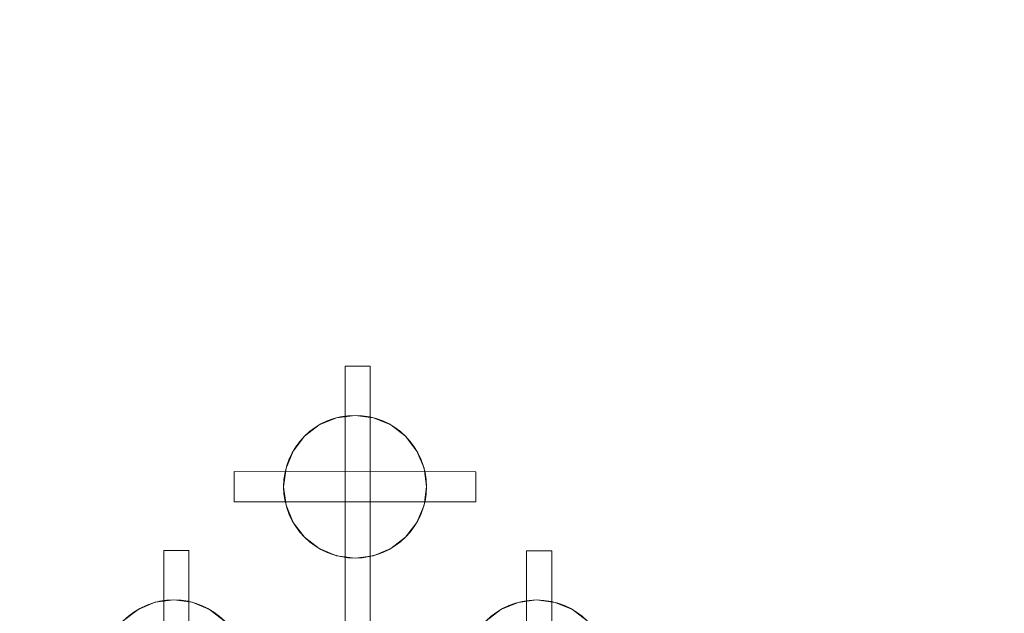
# Model space of a CAD drawing. Units: inches. Extents: x 2696 to 3240, y 1564 to 2310.
# Tile 71 of 76: x 3144.26 to 3156.48, y 2078.13 to 2085.5. Entities that reach past the tile are written whole.
import ezdxf

# ---------------------------------------------------------------- set-up
doc = ezdxf.new("R2010")
doc.units = ezdxf.units.IN
for name, color, linetype, lineweight in [('A-ANNO-DIMS', 3, 'Continuous', 18), ('A-FLOR-FIXT', 8, 'Continuous', 18), ('A-FURN', 251, 'Continuous', 13)]:
    doc.layers.add(name, color=color, linetype=linetype, lineweight=lineweight)
doc.layers.add('FURNITURE', color=250, linetype='Continuous')
doc.styles.add('TIMES NEW', font='times.ttf')
doc.dimstyles.new('Siddhuu', dxfattribs={"dimtxt": 6, "dimasz": 2.5, "dimexe": 1.25, "dimexo": 0.625, "dimtad": 1, "dimdec": 1, "dimlunit": 4, "dimtxsty": 'TIMES NEW', "dimcen": 2.5, "dimclrd": 256, "dimclre": 1, "dimclrt": 7, "dimadec": 0, "dimazin": 0, "dimtfac": 1, "dimtdec": 1, "dimtmove": 0, "dimatfit": 3, "dimfxl": 1, "dimtolj": 1, "dimlwd": -1, "dimarcsym": 0})

# ---------------------------------------------------------------- blocks, each defined once
blk = doc.blocks.new('A$C1af1f523')
at = {"layer": 'A-FURN'}
for p, q in [((-2.9, 3.935), (-2.9, 0.936)), ((-2.9, 3.935, 0.5), (-2.9, 0.936, 0.5)), ((-2.9, 3.935), (-2.9, 3.935, 0.5)), ((-2.525, 3.935), (-2.9, 3.935)), ((-2.525, 3.935, 0.5), (-2.9, 3.935, 0.5)), ((-2.525, 3.935), (-2.525, 0.936)), ((-2.525, 3.935, 0.5), (-2.525, 0.936, 0.5)), ((-2.525, 3.935), (-2.525, 3.935, 0.5)), ((-2.713, 3.321), (-2.713, 3.321, 0.5)), ((-3.156, 3.203), (-3.156, 3.203, 0.5)), ((-2.942, 3.291), (-2.942, 3.291, 0.5)), ((-2.483, 3.291), (-2.483, 3.291, 0.5)), ((-2.27, 3.203), (-2.27, 3.203, 0.5)), ((-3.339, 3.062), (-3.339, 3.062, 0.5)), ((-2.086, 3.062), (-2.086, 3.062, 0.5)), ((-3.48, 2.878), (-3.48, 2.878, 0.5)), ((-1.945, 2.878), (-1.945, 2.878, 0.5)), ((-3.569, 2.665), (-3.569, 2.665, 0.5)), ((-1.857, 2.665), (-1.857, 2.665, 0.5)), ((0, 2.56), (-4.212, 2.56)), ((0, 2.56, 0.5), (-4.212, 2.56, 0.5)), ((-4.212, 2.56), (-4.212, 2.56, 0.5)), ((-4.212, 2.559), (-4.212, 2.248)), ((-4.212, 2.559, 0.5), (-4.212, 2.248, 0.5)), ((-4.212, 2.559), (-4.212, 2.559, 0.5)), ((-3.599, 2.435), (-3.599, 2.435, 0.5)), ((-1.827, 2.435), (-1.827, 2.435, 0.5)), ((0, 2.248), (-4.212, 2.248)), ((0, 2.248, 0.5), (-4.212, 2.248, 0.5)), ((-4.212, 2.248), (-4.212, 2.248, 0.5)), ((-4.212, 2.248), (-4.212, 2.247)), ((-4.212, 2.248, 0.5), (-4.212, 2.247, 0.5)), ((-4.212, 2.247), (-4.212, 2.247, 0.5)), ((-3.569, 2.206), (-3.569, 2.206, 0.5)), ((-1.857, 2.206), (-1.857, 2.206, 0.5)), ((-3.48, 1.992), (-3.48, 1.992, 0.5)), ((-1.945, 1.992), (-1.945, 1.992, 0.5)), ((-3.339, 1.809), (-3.339, 1.809, 0.5)), ((-2.086, 1.809), (-2.086, 1.809, 0.5)), ((-4.816, 1.687), (-5.191, 1.687)), ((-4.816, 1.687, 0.5), (-5.191, 1.687, 0.5)), ((-5.191, 1.687), (-5.191, 1.687, 0.5)), ((-5.191, 1.687), (-5.19, -1.311)), ((-5.191, 1.687, 0.5), (-5.19, -1.311, 0.5)), ((-4.816, 1.687), (-4.816, 1.687, 0.5)), ((-4.816, 1.687), (-4.815, -1.311)), ((-4.816, 1.687, 0.5), (-4.815, -1.311, 0.5)), ((-3.156, 1.668), (-3.156, 1.668, 0.5)), ((-2.27, 1.668), (-2.27, 1.668, 0.5)), ((-2.942, 1.58), (-2.942, 1.58, 0.5)), ((-2.713, 1.549), (-2.713, 1.549, 0.5)), ((-2.483, 1.58), (-2.483, 1.58, 0.5)), ((-5.232, 1.043), (-5.232, 1.043, 0.5)), ((-5.003, 1.074), (-5.003, 1.074, 0.5)), ((-4.773, 1.043), (-4.773, 1.043, 0.5)), ((-5.446, 0.955), (-5.446, 0.955, 0.5)), ((-4.56, 0.955), (-4.56, 0.955, 0.5)), ((-2.9, 0.936), (-2.9, 0.936, 0.5)), ((-2.525, 0.936), (-2.898, 0.936)), ((-2.525, 0.936, 0.5), (-2.898, 0.936, 0.5)), ((-2.898, 0.936), (-2.898, 0.936, 0.5)), ((-2.525, 0.936), (-2.525, 0.936, 0.5)), ((-5.629, 0.814), (-5.629, 0.814, 0.5)), ((-4.376, 0.814), (-4.376, 0.814, 0.5)), ((-5.77, 0.631), (-5.77, 0.631, 0.5)), ((-4.235, 0.631), (-4.235, 0.631, 0.5)), ((-5.858, 0.417), (-5.858, 0.417, 0.5)), ((-4.147, 0.417), (-4.147, 0.417, 0.5)), ((0, 0.312), (-6.501, 0.312)), ((0, 0.312, 0.5), (-6.501, 0.312, 0.5)), ((-6.501, 0.312), (-6.501, 0.312, 0.5)), ((-6.501, 0.311), (-6.501, 0)), ((-6.501, 0.311, 0.5), (-6.501, 0, 0.5)), ((-6.501, 0.311), (-6.501, 0.311, 0.5)), ((-5.889, 0.188), (-5.889, 0.188, 0.5)), ((-4.117, 0.188), (-4.117, 0.188, 0.5)), ((0, 0), (-6.501, 0)), ((0, 0, 0.5), (-6.501, 0, 0.5)), ((-6.501, 0), (-6.501, 0, 0.5)), ((-6.501, 0), (-6.501, -0.001)), ((-6.501, 0, 0.5), (-6.501, -0.001, 0.5)), ((-6.501, -0.001), (-6.501, -0.001, 0.5)), ((-5.858, -0.042), (-5.858, -0.042, 0.5)), ((-4.147, -0.042), (-4.147, -0.042, 0.5)), ((-5.77, -0.256), (-5.77, -0.256, 0.5)), ((-4.235, -0.256), (-4.235, -0.256, 0.5)), ((-5.629, -0.439), (-5.629, -0.439, 0.5)), ((-4.376, -0.439), (-4.376, -0.439, 0.5)), ((-5.446, -0.58), (-5.446, -0.58, 0.5)), ((-4.56, -0.58), (-4.56, -0.58, 0.5)), ((-2.898, -0.564), (-2.898, -3.563)), ((-2.898, -0.564, 0.5), (-2.898, -3.563, 0.5)), ((-2.898, -0.564), (-2.898, -0.564, 0.5)), ((-2.523, -0.564), (-2.898, -0.564)), ((-2.523, -0.564, 0.5), (-2.898, -0.564, 0.5)), ((-2.523, -0.564), (-2.523, -3.563)), ((-2.523, -0.564, 0.5), (-2.523, -3.563, 0.5)), ((-2.523, -0.564), (-2.523, -0.564, 0.5)), ((-5.232, -0.668), (-5.232, -0.668, 0.5)), ((-5.003, -0.699), (-5.003, -0.699, 0.5)), ((-4.773, -0.668), (-4.773, -0.668, 0.5)), ((-2.94, -1.208), (-2.94, -1.208, 0.5)), ((-2.711, -1.178), (-2.711, -1.178, 0.5)), ((-2.481, -1.208), (-2.481, -1.208, 0.5)), ((-5.19, -1.311), (-5.19, -1.311, 0.5)), ((-4.815, -1.311), (-5.188, -1.311)), ((-4.815, -1.311, 0.5), (-5.188, -1.311, 0.5)), ((-5.188, -1.311), (-5.188, -1.311, 0.5)), ((-4.815, -1.311), (-4.815, -1.311, 0.5)), ((-3.154, -1.296), (-3.154, -1.296, 0.5)), ((-2.268, -1.296), (-2.268, -1.296, 0.5)), ((-3.337, -1.437), (-3.337, -1.437, 0.5)), ((-2.084, -1.437), (-2.084, -1.437, 0.5)), ((-3.478, -1.621), (-3.478, -1.621, 0.5)), ((-1.943, -1.621), (-1.943, -1.621, 0.5)), ((0, -1.939), (-4.209, -1.939)), ((0, -1.939, 0.5), (-4.209, -1.939, 0.5)), ((-4.209, -1.939), (-4.209, -1.939, 0.5)), ((-4.209, -1.94), (-4.209, -2.251)), ((-4.209, -1.94, 0.5), (-4.209, -2.251, 0.5)), ((-4.209, -1.94), (-4.209, -1.94, 0.5)), ((-3.566, -1.834), (-3.566, -1.834, 0.5)), ((-1.855, -1.834), (-1.855, -1.834, 0.5)), ((-3.597, -2.064), (-3.597, -2.064, 0.5)), ((-1.824, -2.064), (-1.824, -2.064, 0.5)), ((0, -2.251), (-4.209, -2.251)), ((0, -2.251, 0.5), (-4.209, -2.251, 0.5)), ((-4.209, -2.251), (-4.209, -2.251, 0.5)), ((-4.209, -2.251), (-4.209, -2.252)), ((-4.209, -2.251, 0.5), (-4.209, -2.252, 0.5)), ((-4.209, -2.252), (-4.209, -2.252, 0.5)), ((-3.566, -2.293), (-3.566, -2.293, 0.5)), ((-1.855, -2.293), (-1.855, -2.293, 0.5)), ((-3.478, -2.507), (-3.478, -2.507, 0.5)), ((-1.943, -2.507), (-1.943, -2.507, 0.5)), ((-3.337, -2.69), (-3.337, -2.69, 0.5)), ((-2.084, -2.69), (-2.084, -2.69, 0.5)), ((-3.154, -2.831), (-3.154, -2.831, 0.5)), ((-2.94, -2.92), (-2.94, -2.92, 0.5)), ((-2.481, -2.92), (-2.481, -2.92, 0.5)), ((-2.268, -2.831), (-2.268, -2.831, 0.5)), ((-2.711, -2.95), (-2.711, -2.95, 0.5)), ((-2.898, -3.563), (-2.898, -3.563, 0.5)), ((-2.523, -3.563), (-2.896, -3.563)), ((-2.523, -3.563, 0.5), (-2.896, -3.563, 0.5)), ((-2.896, -3.563), (-2.896, -3.563, 0.5)), ((-2.523, -3.563), (-2.523, -3.563, 0.5))]:
    blk.add_line(p, q, dxfattribs=at)
for centre in [(-2.713, 2.435), (-2.713, 2.435, 0.5), (-5.003, 0.188), (-5.003, 0.188, 0.5), (-2.711, -2.064), (-2.711, -2.064, 0.5)]:
    blk.add_circle(centre, 0.886, dxfattribs=at)
at = {"layer": 'FURNITURE'}
for p, q in [((0, 2.56), (0, 2.56, 0.5)), ((0, 2.248), (0, 2.248, 0.5)), ((0, 0.312), (0, 0.312, 0.5)), ((0, 0), (0, 0, 0.5)), ((0, -1.939), (0, -1.939, 0.5)), ((0, -2.251), (0, -2.251, 0.5))]:
    blk.add_line(p, q, dxfattribs=at)
at = {"layer": 'A-FURN'}
mesh = blk.add_polyface(dxfattribs=at)
corners = [(-2.9, 0.936, 0.5), (-2.9, 3.935), (-2.9, 0.936), (-2.9, 3.935, 0.5)]
mesh.append_faces([[corners[k] for k in face] for face in [(2, 1, 0), (3, 0, 1)]], dxfattribs={"vtx1": -1})
mesh = blk.add_polyface(dxfattribs=at)
corners = [(-2.525, 3.935, 0.5), (-2.9, 3.935), (-2.9, 3.935, 0.5), (-2.525, 3.935)]
mesh.append_faces([[corners[k] for k in face] for face in [(2, 1, 0), (3, 0, 1)]], dxfattribs={"vtx1": -1})
mesh = blk.add_polyface(dxfattribs=at)
corners = [(-2.525, 0.936, 0.5), (-2.525, 3.935), (-2.525, 0.936), (-2.525, 3.935, 0.5)]
mesh.append_faces([[corners[k] for k in face] for face in [(2, 1, 0), (3, 0, 1)]], dxfattribs={"vtx1": -1})
mesh = blk.add_polyface(dxfattribs=at)
corners = [(-2.713, 3.321), (-2.942, 3.291, 0.5), (-2.942, 3.291), (-2.713, 3.321, 0.5)]
mesh.append_faces([[corners[k] for k in face] for face in [(2, 1, 0), (3, 0, 1)]], dxfattribs={"vtx1": -1})
mesh = blk.add_polyface(dxfattribs=at)
corners = [(-2.483, 3.291), (-2.713, 3.321, 0.5), (-2.713, 3.321), (-2.483, 3.291, 0.5)]
mesh.append_faces([[corners[k] for k in face] for face in [(2, 1, 0), (3, 0, 1)]], dxfattribs={"vtx1": -1})
mesh = blk.add_polyface(dxfattribs=at)
corners = [(-3.156, 3.203), (-3.339, 3.062, 0.5), (-3.339, 3.062), (-3.156, 3.203, 0.5)]
mesh.append_faces([[corners[k] for k in face] for face in [(2, 1, 0), (3, 0, 1)]], dxfattribs={"vtx1": -1})
mesh = blk.add_polyface(dxfattribs=at)
corners = [(-2.942, 3.291), (-3.156, 3.203, 0.5), (-3.156, 3.203), (-2.942, 3.291, 0.5)]
mesh.append_faces([[corners[k] for k in face] for face in [(2, 1, 0), (3, 0, 1)]], dxfattribs={"vtx1": -1})
mesh = blk.add_polyface(dxfattribs=at)
corners = [(-2.27, 3.203), (-2.483, 3.291, 0.5), (-2.483, 3.291), (-2.27, 3.203, 0.5)]
mesh.append_faces([[corners[k] for k in face] for face in [(2, 1, 0), (3, 0, 1)]], dxfattribs={"vtx1": -1})
mesh = blk.add_polyface(dxfattribs=at)
corners = [(-2.086, 3.062), (-2.27, 3.203, 0.5), (-2.27, 3.203), (-2.086, 3.062, 0.5)]
mesh.append_faces([[corners[k] for k in face] for face in [(2, 1, 0), (3, 0, 1)]], dxfattribs={"vtx1": -1})
mesh = blk.add_polyface(dxfattribs=at)
corners = [(-3.339, 3.062, 0.5), (-3.48, 2.878), (-3.339, 3.062), (-3.48, 2.878, 0.5)]
mesh.append_faces([[corners[k] for k in face] for face in [(2, 1, 0), (3, 0, 1)]], dxfattribs={"vtx1": -1})
mesh = blk.add_polyface(dxfattribs=at)
corners = [(-1.945, 2.878, 0.5), (-2.086, 3.062), (-1.945, 2.878), (-2.086, 3.062, 0.5)]
mesh.append_faces([[corners[k] for k in face] for face in [(2, 1, 0), (3, 0, 1)]], dxfattribs={"vtx1": -1})
mesh = blk.add_polyface(dxfattribs=at)
corners = [(-3.48, 2.878, 0.5), (-3.569, 2.665), (-3.48, 2.878), (-3.569, 2.665, 0.5)]
mesh.append_faces([[corners[k] for k in face] for face in [(2, 1, 0), (3, 0, 1)]], dxfattribs={"vtx1": -1})
mesh = blk.add_polyface(dxfattribs=at)
corners = [(-1.857, 2.665, 0.5), (-1.945, 2.878), (-1.857, 2.665), (-1.945, 2.878, 0.5)]
mesh.append_faces([[corners[k] for k in face] for face in [(2, 1, 0), (3, 0, 1)]], dxfattribs={"vtx1": -1})
mesh = blk.add_polyface(dxfattribs=at)
corners = [(-3.569, 2.665, 0.5), (-3.599, 2.435), (-3.569, 2.665), (-3.599, 2.435, 0.5)]
mesh.append_faces([[corners[k] for k in face] for face in [(2, 1, 0), (3, 0, 1)]], dxfattribs={"vtx1": -1})
mesh = blk.add_polyface(dxfattribs=at)
corners = [(-1.827, 2.435, 0.5), (-1.857, 2.665), (-1.827, 2.435), (-1.857, 2.665, 0.5)]
mesh.append_faces([[corners[k] for k in face] for face in [(2, 1, 0), (3, 0, 1)]], dxfattribs={"vtx1": -1})
mesh = blk.add_polyface(dxfattribs=at)
corners = [(0, 2.56, 0.5), (-4.212, 2.56), (-4.212, 2.56, 0.5), (0, 2.56)]
mesh.append_faces([[corners[k] for k in face] for face in [(2, 1, 0), (3, 0, 1)]], dxfattribs={"vtx1": -1})
mesh = blk.add_polyface(dxfattribs=at)
corners = [(-4.212, 2.247, 0.5), (-4.212, 2.248), (-4.212, 2.247), (-4.212, 2.559), (-4.212, 2.559, 0.5), (-4.212, 2.248, 0.5)]
mesh.append_faces([[corners[k] for k in face] for face in [(3, 0, 1), (4, 0, 3)]], dxfattribs={"vtx0": -1, "vtx1": -1})
mesh.append_faces([[corners[k] for k in face] for face in [(2, 1, 0), (5, 0, 4)]], dxfattribs={"vtx1": -1})
mesh = blk.add_polyface(dxfattribs=at)
corners = [(-3.599, 2.435, 0.5), (-3.569, 2.206), (-3.599, 2.435), (-3.569, 2.206, 0.5)]
mesh.append_faces([[corners[k] for k in face] for face in [(2, 1, 0), (3, 0, 1)]], dxfattribs={"vtx1": -1})
mesh = blk.add_polyface(dxfattribs=at)
corners = [(-1.857, 2.206, 0.5), (-1.827, 2.435), (-1.857, 2.206), (-1.827, 2.435, 0.5)]
mesh.append_faces([[corners[k] for k in face] for face in [(2, 1, 0), (3, 0, 1)]], dxfattribs={"vtx1": -1})
mesh = blk.add_polyface(dxfattribs=at)
corners = [(0, 2.248, 0.5), (-4.212, 2.248), (-4.212, 2.248, 0.5), (0, 2.248)]
mesh.append_faces([[corners[k] for k in face] for face in [(2, 1, 0), (3, 0, 1)]], dxfattribs={"vtx1": -1})
mesh = blk.add_polyface(dxfattribs=at)
corners = [(-3.569, 2.206, 0.5), (-3.48, 1.992), (-3.569, 2.206), (-3.48, 1.992, 0.5)]
mesh.append_faces([[corners[k] for k in face] for face in [(2, 1, 0), (3, 0, 1)]], dxfattribs={"vtx1": -1})
mesh = blk.add_polyface(dxfattribs=at)
corners = [(-1.945, 1.992, 0.5), (-1.857, 2.206), (-1.945, 1.992), (-1.857, 2.206, 0.5)]
mesh.append_faces([[corners[k] for k in face] for face in [(2, 1, 0), (3, 0, 1)]], dxfattribs={"vtx1": -1})
mesh = blk.add_polyface(dxfattribs=at)
corners = [(-3.48, 1.992, 0.5), (-3.339, 1.809), (-3.48, 1.992), (-3.339, 1.809, 0.5)]
mesh.append_faces([[corners[k] for k in face] for face in [(2, 1, 0), (3, 0, 1)]], dxfattribs={"vtx1": -1})
mesh = blk.add_polyface(dxfattribs=at)
corners = [(-2.086, 1.809, 0.5), (-1.945, 1.992), (-2.086, 1.809), (-1.945, 1.992, 0.5)]
mesh.append_faces([[corners[k] for k in face] for face in [(2, 1, 0), (3, 0, 1)]], dxfattribs={"vtx1": -1})
mesh = blk.add_polyface(dxfattribs=at)
corners = [(-3.156, 1.668, 0.5), (-3.339, 1.809), (-3.339, 1.809, 0.5), (-3.156, 1.668)]
mesh.append_faces([[corners[k] for k in face] for face in [(2, 1, 0), (3, 0, 1)]], dxfattribs={"vtx1": -1})
mesh = blk.add_polyface(dxfattribs=at)
corners = [(-2.086, 1.809, 0.5), (-2.27, 1.668), (-2.27, 1.668, 0.5), (-2.086, 1.809)]
mesh.append_faces([[corners[k] for k in face] for face in [(2, 1, 0), (3, 0, 1)]], dxfattribs={"vtx1": -1})
mesh = blk.add_polyface(dxfattribs=at)
corners = [(-4.816, 1.687, 0.5), (-5.191, 1.687), (-5.191, 1.687, 0.5), (-4.816, 1.687)]
mesh.append_faces([[corners[k] for k in face] for face in [(2, 1, 0), (3, 0, 1)]], dxfattribs={"vtx1": -1})
mesh = blk.add_polyface(dxfattribs=at)
corners = [(-5.19, -1.311, 0.5), (-5.191, 1.687), (-5.19, -1.311), (-5.191, 1.687, 0.5)]
mesh.append_faces([[corners[k] for k in face] for face in [(2, 1, 0), (3, 0, 1)]], dxfattribs={"vtx1": -1})
mesh = blk.add_polyface(dxfattribs=at)
corners = [(-4.815, -1.311, 0.5), (-4.816, 1.687), (-4.815, -1.311), (-4.816, 1.687, 0.5)]
mesh.append_faces([[corners[k] for k in face] for face in [(2, 1, 0), (3, 0, 1)]], dxfattribs={"vtx1": -1})
mesh = blk.add_polyface(dxfattribs=at)
corners = [(-2.942, 1.58, 0.5), (-3.156, 1.668), (-3.156, 1.668, 0.5), (-2.942, 1.58)]
mesh.append_faces([[corners[k] for k in face] for face in [(2, 1, 0), (3, 0, 1)]], dxfattribs={"vtx1": -1})
mesh = blk.add_polyface(dxfattribs=at)
corners = [(-2.27, 1.668, 0.5), (-2.483, 1.58), (-2.483, 1.58, 0.5), (-2.27, 1.668)]
mesh.append_faces([[corners[k] for k in face] for face in [(2, 1, 0), (3, 0, 1)]], dxfattribs={"vtx1": -1})
mesh = blk.add_polyface(dxfattribs=at)
corners = [(-2.713, 1.549, 0.5), (-2.942, 1.58), (-2.942, 1.58, 0.5), (-2.713, 1.549)]
mesh.append_faces([[corners[k] for k in face] for face in [(2, 1, 0), (3, 0, 1)]], dxfattribs={"vtx1": -1})
mesh = blk.add_polyface(dxfattribs=at)
corners = [(-2.483, 1.58, 0.5), (-2.713, 1.549), (-2.713, 1.549, 0.5), (-2.483, 1.58)]
mesh.append_faces([[corners[k] for k in face] for face in [(2, 1, 0), (3, 0, 1)]], dxfattribs={"vtx1": -1})
mesh = blk.add_polyface(dxfattribs=at)
corners = [(-5.232, 1.043), (-5.446, 0.955, 0.5), (-5.446, 0.955), (-5.232, 1.043, 0.5)]
mesh.append_faces([[corners[k] for k in face] for face in [(2, 1, 0), (3, 0, 1)]], dxfattribs={"vtx1": -1})
mesh = blk.add_polyface(dxfattribs=at)
corners = [(-5.003, 1.074), (-5.232, 1.043, 0.5), (-5.232, 1.043), (-5.003, 1.074, 0.5)]
mesh.append_faces([[corners[k] for k in face] for face in [(2, 1, 0), (3, 0, 1)]], dxfattribs={"vtx1": -1})
mesh = blk.add_polyface(dxfattribs=at)
corners = [(-4.773, 1.043), (-5.003, 1.074, 0.5), (-5.003, 1.074), (-4.773, 1.043, 0.5)]
mesh.append_faces([[corners[k] for k in face] for face in [(2, 1, 0), (3, 0, 1)]], dxfattribs={"vtx1": -1})
mesh = blk.add_polyface(dxfattribs=at)
corners = [(-4.56, 0.955), (-4.773, 1.043, 0.5), (-4.773, 1.043), (-4.56, 0.955, 0.5)]
mesh.append_faces([[corners[k] for k in face] for face in [(2, 1, 0), (3, 0, 1)]], dxfattribs={"vtx1": -1})
mesh = blk.add_polyface(dxfattribs=at)
corners = [(-5.446, 0.955), (-5.629, 0.814, 0.5), (-5.629, 0.814), (-5.446, 0.955, 0.5)]
mesh.append_faces([[corners[k] for k in face] for face in [(2, 1, 0), (3, 0, 1)]], dxfattribs={"vtx1": -1})
mesh = blk.add_polyface(dxfattribs=at)
corners = [(-4.376, 0.814), (-4.56, 0.955, 0.5), (-4.56, 0.955), (-4.376, 0.814, 0.5)]
mesh.append_faces([[corners[k] for k in face] for face in [(2, 1, 0), (3, 0, 1)]], dxfattribs={"vtx1": -1})
mesh = blk.add_polyface(dxfattribs=at)
corners = [(-2.525, 0.936, 0.5), (-2.898, 0.936), (-2.898, 0.936, 0.5), (-2.525, 0.936)]
mesh.append_faces([[corners[k] for k in face] for face in [(2, 1, 0), (3, 0, 1)]], dxfattribs={"vtx1": -1})
mesh = blk.add_polyface(dxfattribs=at)
corners = [(-5.629, 0.814, 0.5), (-5.77, 0.631), (-5.629, 0.814), (-5.77, 0.631, 0.5)]
mesh.append_faces([[corners[k] for k in face] for face in [(2, 1, 0), (3, 0, 1)]], dxfattribs={"vtx1": -1})
mesh = blk.add_polyface(dxfattribs=at)
corners = [(-4.235, 0.631, 0.5), (-4.376, 0.814), (-4.235, 0.631), (-4.376, 0.814, 0.5)]
mesh.append_faces([[corners[k] for k in face] for face in [(2, 1, 0), (3, 0, 1)]], dxfattribs={"vtx1": -1})
mesh = blk.add_polyface(dxfattribs=at)
corners = [(-5.77, 0.631, 0.5), (-5.858, 0.417), (-5.77, 0.631), (-5.858, 0.417, 0.5)]
mesh.append_faces([[corners[k] for k in face] for face in [(2, 1, 0), (3, 0, 1)]], dxfattribs={"vtx1": -1})
mesh = blk.add_polyface(dxfattribs=at)
corners = [(-4.147, 0.417, 0.5), (-4.235, 0.631), (-4.147, 0.417), (-4.235, 0.631, 0.5)]
mesh.append_faces([[corners[k] for k in face] for face in [(2, 1, 0), (3, 0, 1)]], dxfattribs={"vtx1": -1})
mesh = blk.add_polyface(dxfattribs=at)
corners = [(-5.858, 0.417, 0.5), (-5.889, 0.188), (-5.858, 0.417), (-5.889, 0.188, 0.5)]
mesh.append_faces([[corners[k] for k in face] for face in [(2, 1, 0), (3, 0, 1)]], dxfattribs={"vtx1": -1})
mesh = blk.add_polyface(dxfattribs=at)
corners = [(-4.117, 0.188, 0.5), (-4.147, 0.417), (-4.117, 0.188), (-4.147, 0.417, 0.5)]
mesh.append_faces([[corners[k] for k in face] for face in [(2, 1, 0), (3, 0, 1)]], dxfattribs={"vtx1": -1})
mesh = blk.add_polyface(dxfattribs=at)
corners = [(0, 0.312, 0.5), (-6.501, 0.312), (-6.501, 0.312, 0.5), (0, 0.312)]
mesh.append_faces([[corners[k] for k in face] for face in [(2, 1, 0), (3, 0, 1)]], dxfattribs={"vtx1": -1})
mesh = blk.add_polyface(dxfattribs=at)
corners = [(-6.501, -0.001, 0.5), (-6.501, 0), (-6.501, -0.001), (-6.501, 0.311), (-6.501, 0.311, 0.5), (-6.501, 0, 0.5)]
mesh.append_faces([[corners[k] for k in face] for face in [(3, 0, 1), (4, 0, 3)]], dxfattribs={"vtx0": -1, "vtx1": -1})
mesh.append_faces([[corners[k] for k in face] for face in [(2, 1, 0), (5, 0, 4)]], dxfattribs={"vtx1": -1})
mesh = blk.add_polyface(dxfattribs=at)
corners = [(-5.889, 0.188, 0.5), (-5.858, -0.042), (-5.889, 0.188), (-5.858, -0.042, 0.5)]
mesh.append_faces([[corners[k] for k in face] for face in [(2, 1, 0), (3, 0, 1)]], dxfattribs={"vtx1": -1})
mesh = blk.add_polyface(dxfattribs=at)
corners = [(-4.147, -0.042, 0.5), (-4.117, 0.188), (-4.147, -0.042), (-4.117, 0.188, 0.5)]
mesh.append_faces([[corners[k] for k in face] for face in [(2, 1, 0), (3, 0, 1)]], dxfattribs={"vtx1": -1})
mesh = blk.add_polyface(dxfattribs=at)
corners = [(0, 0, 0.5), (-6.501, 0), (-6.501, 0, 0.5), (0, 0)]
mesh.append_faces([[corners[k] for k in face] for face in [(2, 1, 0), (3, 0, 1)]], dxfattribs={"vtx1": -1})
mesh = blk.add_polyface(dxfattribs=at)
corners = [(-5.858, -0.042, 0.5), (-5.77, -0.256), (-5.858, -0.042), (-5.77, -0.256, 0.5)]
mesh.append_faces([[corners[k] for k in face] for face in [(2, 1, 0), (3, 0, 1)]], dxfattribs={"vtx1": -1})
mesh = blk.add_polyface(dxfattribs=at)
corners = [(-4.235, -0.256, 0.5), (-4.147, -0.042), (-4.235, -0.256), (-4.147, -0.042, 0.5)]
mesh.append_faces([[corners[k] for k in face] for face in [(2, 1, 0), (3, 0, 1)]], dxfattribs={"vtx1": -1})
mesh = blk.add_polyface(dxfattribs=at)
corners = [(-5.77, -0.256, 0.5), (-5.629, -0.439), (-5.77, -0.256), (-5.629, -0.439, 0.5)]
mesh.append_faces([[corners[k] for k in face] for face in [(2, 1, 0), (3, 0, 1)]], dxfattribs={"vtx1": -1})
mesh = blk.add_polyface(dxfattribs=at)
corners = [(-4.376, -0.439, 0.5), (-4.235, -0.256), (-4.376, -0.439), (-4.235, -0.256, 0.5)]
mesh.append_faces([[corners[k] for k in face] for face in [(2, 1, 0), (3, 0, 1)]], dxfattribs={"vtx1": -1})
mesh = blk.add_polyface(dxfattribs=at)
corners = [(-5.446, -0.58, 0.5), (-5.629, -0.439), (-5.629, -0.439, 0.5), (-5.446, -0.58)]
mesh.append_faces([[corners[k] for k in face] for face in [(2, 1, 0), (3, 0, 1)]], dxfattribs={"vtx1": -1})
mesh = blk.add_polyface(dxfattribs=at)
corners = [(-4.376, -0.439, 0.5), (-4.56, -0.58), (-4.56, -0.58, 0.5), (-4.376, -0.439)]
mesh.append_faces([[corners[k] for k in face] for face in [(2, 1, 0), (3, 0, 1)]], dxfattribs={"vtx1": -1})
mesh = blk.add_polyface(dxfattribs=at)
corners = [(-5.232, -0.668, 0.5), (-5.446, -0.58), (-5.446, -0.58, 0.5), (-5.232, -0.668)]
mesh.append_faces([[corners[k] for k in face] for face in [(2, 1, 0), (3, 0, 1)]], dxfattribs={"vtx1": -1})
mesh = blk.add_polyface(dxfattribs=at)
corners = [(-4.56, -0.58, 0.5), (-4.773, -0.668), (-4.773, -0.668, 0.5), (-4.56, -0.58)]
mesh.append_faces([[corners[k] for k in face] for face in [(2, 1, 0), (3, 0, 1)]], dxfattribs={"vtx1": -1})
mesh = blk.add_polyface(dxfattribs=at)
corners = [(-2.898, -3.563, 0.5), (-2.898, -0.564), (-2.898, -3.563), (-2.898, -0.564, 0.5)]
mesh.append_faces([[corners[k] for k in face] for face in [(2, 1, 0), (3, 0, 1)]], dxfattribs={"vtx1": -1})
mesh = blk.add_polyface(dxfattribs=at)
corners = [(-2.523, -0.564, 0.5), (-2.898, -0.564), (-2.898, -0.564, 0.5), (-2.523, -0.564)]
mesh.append_faces([[corners[k] for k in face] for face in [(2, 1, 0), (3, 0, 1)]], dxfattribs={"vtx1": -1})
mesh = blk.add_polyface(dxfattribs=at)
corners = [(-2.523, -3.563, 0.5), (-2.523, -0.564), (-2.523, -3.563), (-2.523, -0.564, 0.5)]
mesh.append_faces([[corners[k] for k in face] for face in [(2, 1, 0), (3, 0, 1)]], dxfattribs={"vtx1": -1})
mesh = blk.add_polyface(dxfattribs=at)
corners = [(-5.003, -0.699, 0.5), (-5.232, -0.668), (-5.232, -0.668, 0.5), (-5.003, -0.699)]
mesh.append_faces([[corners[k] for k in face] for face in [(2, 1, 0), (3, 0, 1)]], dxfattribs={"vtx1": -1})
mesh = blk.add_polyface(dxfattribs=at)
corners = [(-4.773, -0.668, 0.5), (-5.003, -0.699), (-5.003, -0.699, 0.5), (-4.773, -0.668)]
mesh.append_faces([[corners[k] for k in face] for face in [(2, 1, 0), (3, 0, 1)]], dxfattribs={"vtx1": -1})
mesh = blk.add_polyface(dxfattribs=at)
corners = [(-2.94, -1.208), (-3.154, -1.296, 0.5), (-3.154, -1.296), (-2.94, -1.208, 0.5)]
mesh.append_faces([[corners[k] for k in face] for face in [(2, 1, 0), (3, 0, 1)]], dxfattribs={"vtx1": -1})
mesh = blk.add_polyface(dxfattribs=at)
corners = [(-2.711, -1.178), (-2.94, -1.208, 0.5), (-2.94, -1.208), (-2.711, -1.178, 0.5)]
mesh.append_faces([[corners[k] for k in face] for face in [(2, 1, 0), (3, 0, 1)]], dxfattribs={"vtx1": -1})
mesh = blk.add_polyface(dxfattribs=at)
corners = [(-2.481, -1.208), (-2.711, -1.178, 0.5), (-2.711, -1.178), (-2.481, -1.208, 0.5)]
mesh.append_faces([[corners[k] for k in face] for face in [(2, 1, 0), (3, 0, 1)]], dxfattribs={"vtx1": -1})
mesh = blk.add_polyface(dxfattribs=at)
corners = [(-2.268, -1.296), (-2.481, -1.208, 0.5), (-2.481, -1.208), (-2.268, -1.296, 0.5)]
mesh.append_faces([[corners[k] for k in face] for face in [(2, 1, 0), (3, 0, 1)]], dxfattribs={"vtx1": -1})
mesh = blk.add_polyface(dxfattribs=at)
corners = [(-4.815, -1.311, 0.5), (-5.188, -1.311), (-5.188, -1.311, 0.5), (-4.815, -1.311)]
mesh.append_faces([[corners[k] for k in face] for face in [(2, 1, 0), (3, 0, 1)]], dxfattribs={"vtx1": -1})
mesh = blk.add_polyface(dxfattribs=at)
corners = [(-3.154, -1.296), (-3.337, -1.437, 0.5), (-3.337, -1.437), (-3.154, -1.296, 0.5)]
mesh.append_faces([[corners[k] for k in face] for face in [(2, 1, 0), (3, 0, 1)]], dxfattribs={"vtx1": -1})
mesh = blk.add_polyface(dxfattribs=at)
corners = [(-2.084, -1.437), (-2.268, -1.296, 0.5), (-2.268, -1.296), (-2.084, -1.437, 0.5)]
mesh.append_faces([[corners[k] for k in face] for face in [(2, 1, 0), (3, 0, 1)]], dxfattribs={"vtx1": -1})
mesh = blk.add_polyface(dxfattribs=at)
corners = [(-3.337, -1.437, 0.5), (-3.478, -1.621), (-3.337, -1.437), (-3.478, -1.621, 0.5)]
mesh.append_faces([[corners[k] for k in face] for face in [(2, 1, 0), (3, 0, 1)]], dxfattribs={"vtx1": -1})
mesh = blk.add_polyface(dxfattribs=at)
corners = [(-1.943, -1.621, 0.5), (-2.084, -1.437), (-1.943, -1.621), (-2.084, -1.437, 0.5)]
mesh.append_faces([[corners[k] for k in face] for face in [(2, 1, 0), (3, 0, 1)]], dxfattribs={"vtx1": -1})
mesh = blk.add_polyface(dxfattribs=at)
corners = [(-3.478, -1.621, 0.5), (-3.566, -1.834), (-3.478, -1.621), (-3.566, -1.834, 0.5)]
mesh.append_faces([[corners[k] for k in face] for face in [(2, 1, 0), (3, 0, 1)]], dxfattribs={"vtx1": -1})
mesh = blk.add_polyface(dxfattribs=at)
corners = [(-1.855, -1.834, 0.5), (-1.943, -1.621), (-1.855, -1.834), (-1.943, -1.621, 0.5)]
mesh.append_faces([[corners[k] for k in face] for face in [(2, 1, 0), (3, 0, 1)]], dxfattribs={"vtx1": -1})
mesh = blk.add_polyface(dxfattribs=at)
corners = [(0, -1.939, 0.5), (-4.209, -1.939), (-4.209, -1.939, 0.5), (0, -1.939)]
mesh.append_faces([[corners[k] for k in face] for face in [(2, 1, 0), (3, 0, 1)]], dxfattribs={"vtx1": -1})
mesh = blk.add_polyface(dxfattribs=at)
corners = [(-4.209, -2.252, 0.5), (-4.209, -2.251), (-4.209, -2.252), (-4.209, -1.94), (-4.209, -1.94, 0.5), (-4.209, -2.251, 0.5)]
mesh.append_faces([[corners[k] for k in face] for face in [(3, 0, 1), (4, 0, 3)]], dxfattribs={"vtx0": -1, "vtx1": -1})
mesh.append_faces([[corners[k] for k in face] for face in [(2, 1, 0), (5, 0, 4)]], dxfattribs={"vtx1": -1})
mesh = blk.add_polyface(dxfattribs=at)
corners = [(-3.566, -1.834, 0.5), (-3.597, -2.064), (-3.566, -1.834), (-3.597, -2.064, 0.5)]
mesh.append_faces([[corners[k] for k in face] for face in [(2, 1, 0), (3, 0, 1)]], dxfattribs={"vtx1": -1})
mesh = blk.add_polyface(dxfattribs=at)
corners = [(-1.824, -2.064, 0.5), (-1.855, -1.834), (-1.824, -2.064), (-1.855, -1.834, 0.5)]
mesh.append_faces([[corners[k] for k in face] for face in [(2, 1, 0), (3, 0, 1)]], dxfattribs={"vtx1": -1})
mesh = blk.add_polyface(dxfattribs=at)
corners = [(-3.597, -2.064, 0.5), (-3.566, -2.293), (-3.597, -2.064), (-3.566, -2.293, 0.5)]
mesh.append_faces([[corners[k] for k in face] for face in [(2, 1, 0), (3, 0, 1)]], dxfattribs={"vtx1": -1})
mesh = blk.add_polyface(dxfattribs=at)
corners = [(-1.855, -2.293, 0.5), (-1.824, -2.064), (-1.855, -2.293), (-1.824, -2.064, 0.5)]
mesh.append_faces([[corners[k] for k in face] for face in [(2, 1, 0), (3, 0, 1)]], dxfattribs={"vtx1": -1})
mesh = blk.add_polyface(dxfattribs=at)
corners = [(0, -2.251, 0.5), (-4.209, -2.251), (-4.209, -2.251, 0.5), (0, -2.251)]
mesh.append_faces([[corners[k] for k in face] for face in [(2, 1, 0), (3, 0, 1)]], dxfattribs={"vtx1": -1})
mesh = blk.add_polyface(dxfattribs=at)
corners = [(-3.566, -2.293, 0.5), (-3.478, -2.507), (-3.566, -2.293), (-3.478, -2.507, 0.5)]
mesh.append_faces([[corners[k] for k in face] for face in [(2, 1, 0), (3, 0, 1)]], dxfattribs={"vtx1": -1})
mesh = blk.add_polyface(dxfattribs=at)
corners = [(-1.943, -2.507, 0.5), (-1.855, -2.293), (-1.943, -2.507), (-1.855, -2.293, 0.5)]
mesh.append_faces([[corners[k] for k in face] for face in [(2, 1, 0), (3, 0, 1)]], dxfattribs={"vtx1": -1})
mesh = blk.add_polyface(dxfattribs=at)
corners = [(-3.478, -2.507, 0.5), (-3.337, -2.69), (-3.478, -2.507), (-3.337, -2.69, 0.5)]
mesh.append_faces([[corners[k] for k in face] for face in [(2, 1, 0), (3, 0, 1)]], dxfattribs={"vtx1": -1})
mesh = blk.add_polyface(dxfattribs=at)
corners = [(-2.084, -2.69, 0.5), (-1.943, -2.507), (-2.084, -2.69), (-1.943, -2.507, 0.5)]
mesh.append_faces([[corners[k] for k in face] for face in [(2, 1, 0), (3, 0, 1)]], dxfattribs={"vtx1": -1})
mesh = blk.add_polyface(dxfattribs=at)
corners = [(-3.154, -2.831, 0.5), (-3.337, -2.69), (-3.337, -2.69, 0.5), (-3.154, -2.831)]
mesh.append_faces([[corners[k] for k in face] for face in [(2, 1, 0), (3, 0, 1)]], dxfattribs={"vtx1": -1})
mesh = blk.add_polyface(dxfattribs=at)
corners = [(-2.084, -2.69, 0.5), (-2.268, -2.831), (-2.268, -2.831, 0.5), (-2.084, -2.69)]
mesh.append_faces([[corners[k] for k in face] for face in [(2, 1, 0), (3, 0, 1)]], dxfattribs={"vtx1": -1})
mesh = blk.add_polyface(dxfattribs=at)
corners = [(-2.94, -2.92, 0.5), (-3.154, -2.831), (-3.154, -2.831, 0.5), (-2.94, -2.92)]
mesh.append_faces([[corners[k] for k in face] for face in [(2, 1, 0), (3, 0, 1)]], dxfattribs={"vtx1": -1})
mesh = blk.add_polyface(dxfattribs=at)
corners = [(-2.711, -2.95, 0.5), (-2.94, -2.92), (-2.94, -2.92, 0.5), (-2.711, -2.95)]
mesh.append_faces([[corners[k] for k in face] for face in [(2, 1, 0), (3, 0, 1)]], dxfattribs={"vtx1": -1})
mesh = blk.add_polyface(dxfattribs=at)
corners = [(-2.481, -2.92, 0.5), (-2.711, -2.95), (-2.711, -2.95, 0.5), (-2.481, -2.92)]
mesh.append_faces([[corners[k] for k in face] for face in [(2, 1, 0), (3, 0, 1)]], dxfattribs={"vtx1": -1})
mesh = blk.add_polyface(dxfattribs=at)
corners = [(-2.268, -2.831, 0.5), (-2.481, -2.92), (-2.481, -2.92, 0.5), (-2.268, -2.831)]
mesh.append_faces([[corners[k] for k in face] for face in [(2, 1, 0), (3, 0, 1)]], dxfattribs={"vtx1": -1})
mesh = blk.add_polyface(dxfattribs=at)
corners = [(-2.523, -3.563, 0.5), (-2.896, -3.563), (-2.896, -3.563, 0.5), (-2.523, -3.563)]
mesh.append_faces([[corners[k] for k in face] for face in [(2, 1, 0), (3, 0, 1)]], dxfattribs={"vtx1": -1})
blk = doc.blocks.new('*D54')
at = {"layer": 'A-ANNO-DIMS', "color": 1, "lineweight": -2, "transparency": 16777216}
for p, q in [((3124.611, 1893.826), (3124.611, 2298.451)), ((3136.611, 1893.826), (3136.611, 2298.451))]:
    blk.add_line(p, q, dxfattribs=at)
at = {"layer": 'A-ANNO-DIMS', "transparency": 16777216}
for p, q in [((3127.111, 2297.201), (3134.111, 2297.201)), ((3136.611, 2297.201), (3155.757, 2297.201))]:
    blk.add_line(p, q, dxfattribs=at)
for points in [[(3127.111, 2297.618), (3127.111, 2296.784), (3124.611, 2297.201)], [(3134.111, 2297.618), (3134.111, 2296.784), (3136.611, 2297.201)]]:
    blk.add_solid(points, dxfattribs=at)
at = {"layer": 'Defpoints', "color": 0, "transparency": 16777216}
for p in [(3136.611, 2297.201), (3124.611, 1893.201), (3136.611, 1893.201)]:
    blk.add_point(p, dxfattribs=at)
at = {"layer": 'A-ANNO-DIMS', "color": 7, "transparency": 16777216, "insert": (3147.434, 2300.878), "char_height": 6, "attachment_point": 5, "style": 'TIMES NEW'}
blk.add_mtext('\\A1;1\'-0"', dxfattribs=at)

msp = doc.modelspace()

# ---------------------------------------------------------------- block references
at = {"layer": 'A-FLOR-FIXT', "xscale": -1, "rotation": 90}
msp.add_blockref('A$C1af1f523', (3148.611, 2074.701), dxfattribs=at)

# ---------------------------------------------------------------- dimensions: what is measured, and where the dimension line sits
at = {"layer": 'A-ANNO-DIMS'}
dim = msp.add_linear_dim(base=(3136.611, 2297.201), p1=(3124.611, 1893.201), p2=(3136.611, 1893.201), dimstyle='Siddhuu', override={"dimdec": 1, "dimlfac": 1, "dimrnd": 0, "dimzin": 1, "dimdsep": 46, "dimlunit": 4, "dimfrac": 2}, dxfattribs=at)
dim.commit()
dim.dimension.update_dxf_attribs({"geometry": '*D54', "text_midpoint": (3147.434, 2300.878)})

doc.saveas('drawing.dxf')
